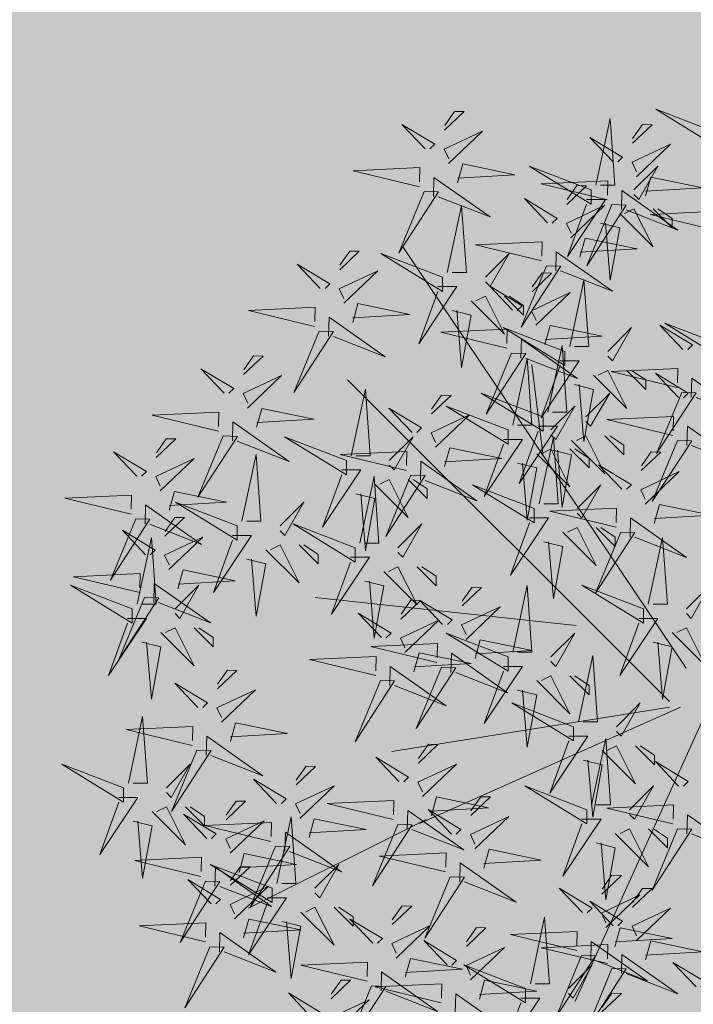
# Model space of a CAD drawing. Units: inches. Extents: x 1704 to 6393, y -157 to 1172.
# Tile 81 of 122: x 2048 to 2064, y 1006 to 1030. Entities that reach past the tile are written whole.
import ezdxf

# ---------------------------------------------------------------- set-up
doc = ezdxf.new("R2010")
doc.units = ezdxf.units.IN
doc.header["$MEASUREMENT"] = 0
doc.layers.add('A-ANNO-DIMS', color=7, linetype='Continuous', lineweight=13)
doc.layers.add('L-shrub', color=74, linetype='Continuous', lineweight=18)
doc.layers.add('L-HRDS-PATT', color=9, linetype='Continuous', lineweight=13, true_color=0xc5c1ba)
doc.styles.get("Standard").update_dxf_attribs({"font": 'arial.ttf'})
doc.dimstyles.get("Standard").update_dxf_attribs({"dimtxt": 6, "dimasz": 2, "dimexe": 0.18, "dimexo": 0.0625, "dimgap": 0.09, "dimtad": 0, "dimtih": 1, "dimtoh": 1, "dimdec": 1, "dimzin": 0, "dimdsep": 46, "dimlunit": 3, "dimtxsty": 'Standard', "dimblk": 'ARCHTICK', "dimcen": 0.09, "dimadec": 0, "dimazin": 0, "dimtfac": 1, "dimtdec": 1, "dimtofl": 0, "dimtmove": 0, "dimatfit": 3, "dimfxl": 1, "dimtolj": 1, "dimtzin": 0, "dimarcsym": 0})

# ---------------------------------------------------------------- blocks, each defined once
blk = doc.blocks.new('shrub3')
for p, q in [((-5.99, -2.5), (58.67, 140.12)), ((130.91, 52.02), (217.13, 95.08)), ((7.48, -2.5), (134.11, 54.01)), ((12.87, -2.5), (147.58, 19.03)), ((12.87, -5.19), (169.14, -161.27)), ((4.78, -21.34), (142.19, -225.85)), ((58.17, -42.16), (184.8, -55.61)), ((74.33, -125.58), (79.72, -168.64))]:
    blk.add_line(p, q)
for points in [[(85.01, 138.66), (75.77, 138.66), (94.24, 166.33), (85.01, 140.97)], [(157.38, 132.76), (169.66, 162.48), (150.47, 132.94), (157.38, 132.76)], [(40.78, 124.29), (53.06, 154.01), (33.87, 124.47), (40.78, 124.29)], [(116.79, 145.77), (116.56, 136.54), (89.36, 155.7), (114.49, 145.83)], [(175.19, 155.2), (158.65, 139.45), (177.32, 148.22), (175.13, 152.89)], [(45.65, 145.34), (36.2, 136.34), (40.81, 136.22), (45.59, 143.03)], [(55.62, 117.94), (67.9, 147.66), (48.71, 118.11), (55.62, 117.94)], [(152.83, 135.19), (152.6, 125.95), (125.4, 145.11), (150.53, 135.24)], [(186.54, 147.99), (197.78, 136.16), (181.88, 145.8), (184.24, 148.05)], [(235.82, 113.71), (248.1, 143.42), (228.91, 113.88), (235.82, 113.71)], [(61.92, 134.05), (50.38, 122.52), (59.61, 138.66), (61.92, 136.35)], [(105.09, 139.14), (102.56, 129.96), (77.32, 135.21), (105.04, 136.83)], [(82.7, 134.05), (112.71, 122.52), (82.7, 140.97), (82.7, 134.05)], [(123.59, 140.98), (155.69, 133.25), (123.36, 131.75), (123.53, 138.68)], [(177.09, 138.99), (167.64, 129.99), (172.25, 129.87), (177.04, 136.68)], [(36.23, 126.72), (36, 117.49), (8.8, 136.64), (33.93, 126.77)], [(-0.02, 133.17), (11.22, 121.34), (-4.68, 130.97), (-2.32, 133.22)], [(51.07, 120.36), (50.84, 111.13), (23.64, 130.29), (48.77, 120.42)], [(80.39, 131.74), (73.46, 99.46), (71.15, 131.74), (78.08, 131.74)], [(109.47, 129.79), (92.93, 114.04), (111.6, 122.81), (109.41, 127.48)], [(159.63, 130.4), (191.73, 122.67), (159.4, 121.17), (159.57, 128.09)], [(201.04, 101.49), (191.81, 103.79), (196.42, 129.16), (198.73, 101.49)], [(141.13, 128.55), (138.6, 119.38), (113.36, 124.63), (141.08, 126.24)], [(231.27, 116.13), (231.04, 106.9), (203.84, 126.05), (228.97, 116.19)], [(24.53, 120.08), (22, 110.91), (-3.24, 116.16), (24.47, 117.77)], [(43.03, 121.93), (75.13, 114.2), (42.8, 112.7), (42.97, 119.62)], [(120.82, 122.58), (132.06, 110.75), (116.16, 120.39), (118.52, 122.64)], [(57.87, 115.58), (89.97, 107.84), (57.64, 106.34), (57.81, 113.27)], [(145.51, 119.2), (128.97, 103.45), (147.64, 112.22), (145.45, 116.9)], [(207.97, 89.96), (198.73, 89.96), (217.2, 117.63), (207.97, 92.27)], [(39.37, 113.73), (36.84, 104.56), (11.6, 109.81), (39.31, 111.42)], [(28.91, 110.73), (12.37, 94.98), (31.04, 103.75), (28.85, 108.43)], [(111.37, 113.58), (101.92, 104.58), (106.53, 104.46), (111.31, 111.27)], [(156.86, 111.99), (168.1, 100.16), (152.2, 109.8), (154.56, 112.05)], [(191.81, 96.88), (175.65, 113.02), (184.88, 94.57), (189.5, 96.88)], [(237.94, 81.95), (250.22, 111.66), (231.03, 82.12), (237.94, 81.95)], [(238.07, 111.34), (270.17, 103.61), (237.84, 102.11), (238.01, 109.03)], [(119.22, 79.83), (131.5, 109.54), (112.31, 80), (119.22, 79.83)], [(219.57, 109.49), (217.04, 100.32), (191.8, 105.57), (219.52, 107.19)], [(43.75, 104.38), (27.21, 88.63), (45.88, 97.4), (43.69, 102.07)], [(40.26, 103.52), (51.5, 91.69), (35.6, 101.33), (37.96, 103.58)], [(147.41, 102.99), (137.96, 93.99), (142.57, 93.88), (147.36, 100.68)], [(175.65, 94.57), (166.41, 103.79), (166.41, 99.18), (173.34, 94.57)], [(55.1, 97.17), (66.34, 85.34), (50.44, 94.98), (52.8, 97.23)], [(223.95, 100.15), (207.41, 84.4), (226.08, 93.17), (223.89, 97.84)], [(30.81, 94.52), (21.36, 85.52), (25.97, 85.41), (30.75, 92.21)], [(48.4, 63.38), (39.16, 65.68), (43.78, 91.04), (46.09, 63.38)], [(114.67, 82.25), (114.44, 73.02), (87.24, 92.18), (112.37, 82.31)], [(204.02, 65.01), (216.3, 94.72), (197.11, 65.18), (204.02, 65.01)], [(205.66, 85.35), (235.67, 73.82), (205.66, 92.27), (205.66, 85.35)], [(233.39, 84.37), (233.16, 75.14), (205.96, 94.29), (231.09, 84.43)], [(235.3, 92.94), (246.54, 81.11), (230.64, 90.74), (233, 92.99)], [(8.98, 56.54), (21.26, 86.25), (2.07, 56.71), (8.98, 56.54)], [(45.65, 88.17), (36.2, 79.17), (40.81, 79.05), (45.59, 85.86)], [(184.88, 85.35), (173.34, 73.82), (182.57, 89.96), (184.88, 87.65)], [(144.66, 54.42), (156.94, 84.13), (137.75, 54.59), (144.66, 54.42)], [(203.35, 83.04), (196.42, 50.76), (194.11, 83.04), (201.04, 83.04)], [(225.85, 83.93), (216.4, 74.93), (221.01, 74.82), (225.8, 81.63)], [(55.33, 51.85), (46.09, 51.85), (64.56, 79.52), (55.33, 54.15)], [(121.47, 77.46), (153.57, 69.73), (121.24, 68.23), (121.41, 75.15)], [(199.47, 67.43), (199.24, 58.2), (172.04, 77.35), (197.17, 67.49)], [(221.69, 77.73), (219.16, 68.56), (193.92, 73.81), (221.64, 75.43)], [(240.19, 79.58), (272.29, 71.85), (239.96, 70.35), (240.13, 77.27)], [(273.12, 52.79), (263.89, 55.09), (268.5, 80.46), (270.81, 52.79)], [(39.16, 58.76), (23, 74.9), (32.24, 56.46), (36.86, 58.76)], [(102.97, 75.62), (100.44, 66.44), (75.2, 71.69), (102.92, 73.31)], [(4.43, 58.96), (4.2, 49.73), (-23, 68.88), (2.13, 59.02)], [(226.07, 68.39), (209.53, 52.64), (228.2, 61.41), (226.01, 66.08)], [(280.05, 41.26), (270.81, 41.26), (289.28, 68.93), (280.05, 43.57)], [(23, 56.46), (13.77, 65.68), (13.77, 61.07), (20.7, 56.46)], [(107.35, 66.27), (90.81, 50.52), (109.48, 59.29), (107.29, 63.96)], [(140.11, 56.84), (139.88, 47.61), (112.68, 66.77), (137.81, 56.9)], [(206.27, 62.64), (238.37, 54.91), (206.04, 53.41), (206.21, 60.33)], [(263.89, 48.18), (247.73, 64.32), (256.96, 45.87), (261.58, 48.18)], [(118.7, 59.06), (129.94, 47.23), (114.04, 56.86), (116.4, 59.12)], [(187.77, 60.79), (185.24, 51.62), (160, 56.87), (187.72, 58.49)], [(237.42, 61.17), (248.66, 49.35), (232.76, 58.98), (235.12, 61.23)], [(11.23, 54.17), (43.33, 46.44), (11, 44.94), (11.17, 51.86)], [(53.02, 47.24), (83.03, 35.71), (53.02, 54.15), (53.02, 47.24)], [(247.73, 45.87), (238.49, 55.09), (238.49, 50.48), (245.42, 45.87)], [(32.24, 47.24), (20.7, 35.71), (29.93, 51.85), (32.24, 49.54)], [(54.76, 23.15), (45.52, 25.45), (50.14, 50.81), (52.45, 23.15)], [(109.25, 50.06), (99.8, 41.06), (104.41, 40.94), (109.19, 47.75)], [(128.41, 50.21), (125.88, 41.03), (100.64, 46.28), (128.36, 47.9)], [(146.91, 52.05), (179.01, 44.32), (146.68, 42.82), (146.85, 49.75)], [(192.15, 51.45), (175.61, 35.7), (194.28, 44.47), (192.09, 49.14)], [(227.97, 52.17), (218.52, 43.17), (223.13, 43.06), (227.92, 49.87)], [(242.18, 18.42), (254.46, 48.14), (235.27, 18.6), (242.18, 18.42)], [(50.71, 44.93), (43.78, 12.65), (41.47, 44.93), (48.4, 44.93)], [(203.5, 44.24), (214.74, 32.41), (198.84, 42.04), (201.2, 44.29)], [(277.74, 36.65), (307.75, 25.12), (277.74, 43.57), (277.74, 36.65)], [(61.69, 11.62), (52.45, 11.62), (70.92, 39.29), (61.69, 13.92)], [(132.79, 40.86), (116.25, 25.11), (134.92, 33.88), (132.73, 38.55)], [(256.96, 36.65), (245.42, 25.12), (254.65, 41.26), (256.96, 38.95)], [(8.46, 35.77), (19.7, 23.94), (3.8, 33.57), (6.16, 35.82)], [(45.52, 18.53), (29.36, 34.67), (38.6, 16.23), (43.22, 18.53)], [(144.14, 33.65), (155.38, 21.82), (139.48, 31.46), (141.84, 33.71)], [(194.05, 35.23), (184.6, 26.23), (189.21, 26.12), (194, 32.93)], [(275.43, 34.34), (268.5, 2.06), (266.19, 34.34), (273.12, 34.34)], [(237.63, 20.85), (237.4, 11.62), (210.2, 30.77), (235.33, 20.91)], [(29.36, 16.23), (20.13, 25.45), (20.13, 20.84), (27.06, 16.23)], [(134.69, 24.65), (125.24, 15.65), (129.85, 15.53), (134.63, 22.34)], [(86.56, -10.73), (77.32, -8.43), (81.94, 16.94), (84.25, -10.73)], [(244.43, 16.06), (276.53, 8.33), (244.2, 6.83), (244.37, 13.75)], [(38.6, 7), (27.06, -4.52), (36.29, 11.62), (38.6, 9.31)], [(59.38, 7), (89.39, -4.52), (59.38, 13.92), (59.38, 7)], [(153.14, -15.45), (165.42, 14.26), (146.23, -15.28), (153.14, -15.45)], [(225.93, 14.21), (223.4, 5.04), (198.16, 10.29), (225.88, 11.9)], [(93.49, -22.26), (84.25, -22.26), (102.72, 5.41), (93.49, -19.96)], [(123.46, -21.81), (135.74, 7.91), (116.55, -21.63), (123.46, -21.81)], [(230.31, 4.87), (213.77, -10.89), (232.44, -2.12), (230.25, 2.56)], [(57.07, 4.7), (50.14, -27.58), (47.83, 4.7), (54.76, 4.7)], [(77.32, -15.34), (61.16, 0.8), (70.4, -17.65), (75.02, -15.34)], [(148.59, -13.03), (148.36, -22.26), (121.16, -3.11), (146.29, -12.97)], [(241.66, -2.35), (252.9, -14.18), (237, -4.54), (239.36, -2.29)], [(20.84, -34.02), (11.6, -31.72), (16.22, -6.36), (18.53, -34.02)], [(61.16, -17.65), (51.93, -8.43), (51.93, -13.04), (58.86, -17.65)], [(118.91, -19.38), (118.68, -28.61), (91.48, -9.46), (116.61, -19.33)], [(268.88, -34.02), (259.65, -31.72), (264.26, -6.36), (266.57, -34.02)], [(232.21, -11.35), (222.76, -20.35), (227.37, -20.46), (232.16, -13.66)], [(27.76, -45.55), (18.53, -45.55), (37, -17.88), (27.76, -43.25)], [(155.39, -17.82), (187.49, -25.55), (155.16, -27.05), (155.33, -20.13)], [(275.81, -45.55), (266.57, -45.55), (285.04, -17.88), (275.81, -43.25)], [(11.6, -38.64), (-4.56, -22.5), (4.68, -40.94), (9.3, -38.64)], [(70.4, -26.87), (58.86, -38.4), (68.09, -22.26), (70.4, -24.57)], [(91.18, -26.87), (121.19, -38.4), (91.18, -19.96), (91.18, -26.87)], [(136.89, -19.67), (134.36, -28.84), (109.12, -23.59), (136.84, -21.97)], [(259.65, -38.64), (243.49, -22.5), (252.72, -40.94), (257.34, -38.64)], [(107.21, -26.02), (104.68, -35.19), (79.44, -29.94), (107.16, -28.33)], [(125.71, -24.17), (157.81, -31.9), (125.48, -33.4), (125.65, -26.48)], [(267.62, -55.68), (279.9, -25.97), (260.71, -55.51), (267.62, -55.68)], [(88.87, -29.18), (81.94, -61.46), (79.63, -29.18), (86.56, -29.18)], [(141.27, -29.01), (124.73, -44.76), (143.4, -35.99), (141.21, -31.32)], [(243.49, -40.94), (234.25, -31.72), (234.25, -36.33), (241.18, -40.94)], [(111.59, -35.37), (95.05, -51.12), (113.72, -42.35), (111.53, -37.67)], [(152.62, -36.23), (163.86, -48.05), (147.96, -38.42), (150.32, -36.17)], [(160.76, -63.67), (151.53, -61.36), (156.14, -36), (158.45, -63.67)], [(122.94, -42.58), (134.18, -54.41), (118.28, -44.77), (120.64, -42.52)], [(4.68, -50.16), (-6.86, -61.69), (2.37, -45.55), (4.68, -47.86)], [(25.46, -50.16), (55.47, -61.69), (25.46, -43.25), (25.46, -50.16)], [(143.17, -45.23), (133.72, -54.23), (138.33, -54.34), (143.12, -47.53)], [(167.69, -75.2), (158.45, -75.2), (176.92, -47.53), (167.69, -72.89)], [(218, -74.25), (208.77, -71.95), (213.38, -46.59), (215.69, -74.25)], [(263.07, -53.26), (262.84, -62.49), (235.64, -43.34), (260.77, -53.2)], [(252.72, -50.16), (241.18, -61.69), (250.41, -45.55), (252.72, -47.86)], [(273.5, -50.16), (303.51, -61.69), (273.5, -43.25), (273.5, -50.16)], [(23.15, -52.47), (16.22, -84.75), (13.91, -52.47), (20.84, -52.47)], [(113.49, -51.58), (104.04, -60.58), (108.65, -60.69), (113.43, -53.89)], [(151.53, -68.28), (135.37, -52.14), (144.6, -70.59), (149.22, -68.28)], [(271.19, -52.47), (264.26, -84.75), (261.95, -52.47), (268.88, -52.47)], [(73.84, -82.72), (64.6, -80.42), (69.22, -55.06), (71.53, -82.72)], [(36.54, -87.45), (48.82, -57.73), (29.63, -87.27), (36.54, -87.45)], [(135.37, -70.59), (126.13, -61.36), (126.13, -65.97), (133.06, -70.59)], [(224.93, -85.78), (215.69, -85.78), (234.16, -58.11), (224.93, -83.48)], [(251.37, -59.9), (248.84, -69.07), (223.6, -63.82), (251.32, -62.2)], [(269.87, -58.05), (301.97, -65.78), (269.64, -67.28), (269.81, -60.36)], [(80.77, -94.25), (71.53, -94.25), (90, -66.58), (80.77, -91.95)], [(208.77, -78.87), (192.61, -62.73), (201.84, -81.17), (206.46, -78.87)], [(271.86, -93.8), (284.14, -64.08), (264.95, -93.62), (271.86, -93.8)], [(64.6, -87.34), (48.44, -71.2), (57.68, -89.64), (62.3, -87.34)], [(255.75, -69.24), (239.21, -85), (257.88, -76.23), (255.7, -71.55)], [(31.99, -85.02), (31.76, -94.25), (4.56, -75.1), (29.69, -84.96)], [(144.6, -79.81), (133.06, -91.34), (142.29, -75.2), (144.6, -77.5)], [(165.38, -79.81), (195.39, -91.34), (165.38, -72.89), (165.38, -79.81)], [(192.61, -81.17), (183.37, -71.95), (183.37, -76.56), (190.3, -81.17)], [(267.1, -76.46), (278.34, -88.28), (262.44, -78.65), (264.8, -76.4)], [(48.44, -89.64), (39.21, -80.42), (39.21, -85.03), (46.14, -89.64)], [(165, -106.02), (155.77, -103.71), (160.38, -78.35), (162.69, -106.02)], [(138.3, -114.97), (150.58, -85.26), (131.39, -114.8), (138.3, -114.97)], [(163.07, -82.11), (156.14, -114.39), (153.83, -82.11), (160.76, -82.11)], [(201.84, -90.4), (190.3, -101.92), (199.53, -85.78), (201.84, -88.09)], [(222.62, -90.4), (252.63, -101.92), (222.62, -83.48), (222.62, -90.4)], [(267.31, -91.37), (267.08, -100.61), (239.88, -81.45), (265.01, -91.32)], [(257.65, -85.46), (248.2, -94.46), (252.81, -94.57), (257.6, -87.76)], [(38.79, -89.81), (70.89, -97.54), (38.56, -99.04), (38.73, -92.12)], [(171.93, -117.54), (162.69, -117.54), (181.16, -89.88), (171.93, -115.24)], [(20.29, -91.66), (17.76, -100.83), (-7.48, -95.58), (20.23, -93.97)], [(57.68, -98.86), (46.14, -110.39), (55.37, -94.25), (57.68, -96.56)], [(86.56, -120.84), (77.32, -118.53), (81.94, -93.17), (84.25, -120.84)], [(78.46, -98.86), (108.47, -110.39), (78.46, -91.95), (78.46, -98.86)], [(155.77, -110.63), (139.61, -94.49), (148.84, -112.93), (153.46, -110.63)], [(220.31, -92.7), (213.38, -124.98), (211.07, -92.7), (218, -92.7)], [(69.6, -127.19), (60.36, -124.88), (64.98, -99.52), (67.29, -127.19)], [(255.61, -98.01), (253.08, -107.18), (227.84, -101.93), (255.56, -100.32)], [(274.11, -96.16), (306.21, -103.89), (273.88, -105.4), (274.05, -98.47)], [(8.98, -131.91), (21.26, -102.2), (2.07, -131.74), (8.98, -131.91)], [(24.67, -101), (8.13, -116.76), (26.8, -107.99), (24.61, -103.31)], [(76.15, -101.17), (69.22, -133.45), (66.91, -101.17), (73.84, -101.17)], [(93.49, -132.37), (84.25, -132.37), (102.72, -104.7), (93.49, -130.06)], [(133.75, -112.55), (133.52, -121.78), (106.32, -102.62), (131.45, -112.49)], [(139.61, -112.93), (130.37, -103.71), (130.37, -108.32), (137.3, -112.93)], [(229.46, -134.03), (241.74, -104.31), (222.55, -133.86), (229.46, -134.03)], [(36.02, -108.22), (47.26, -120.04), (31.36, -110.41), (33.72, -108.16)], [(77.32, -125.45), (61.16, -109.31), (70.4, -127.75), (75.02, -125.45)], [(259.99, -107.36), (243.45, -123.11), (262.12, -114.34), (259.94, -109.66)], [(76.53, -138.72), (67.29, -138.72), (85.76, -111.05), (76.53, -136.41)], [(271.34, -114.57), (282.58, -126.4), (266.68, -116.76), (269.04, -114.51)], [(26.57, -117.22), (17.12, -126.22), (21.73, -126.33), (26.51, -119.53)], [(60.36, -131.8), (44.2, -115.66), (53.44, -134.11), (58.06, -131.8)], [(61.16, -127.75), (51.93, -118.53), (51.93, -123.14), (58.86, -127.75)], [(122.05, -119.18), (119.52, -128.36), (94.28, -123.11), (122, -121.49)], [(148.84, -122.16), (137.3, -133.69), (146.53, -117.54), (148.84, -119.85)], [(140.55, -117.34), (172.65, -125.07), (140.32, -126.57), (140.49, -119.65)], [(169.62, -122.16), (199.63, -133.69), (169.62, -115.24), (169.62, -122.16)], [(4.43, -129.49), (4.2, -138.72), (-23, -119.56), (2.13, -129.43)], [(224.91, -131.61), (224.68, -140.84), (197.48, -121.68), (222.61, -131.55)], [(261.89, -123.57), (252.44, -132.57), (257.05, -132.69), (261.84, -125.88)], [(6.86, -155.2), (19.14, -125.49), (-0.05, -155.03), (6.86, -155.2)], [(44.2, -134.11), (34.97, -124.88), (34.97, -129.5), (41.9, -134.11)], [(126.43, -128.53), (109.89, -144.28), (128.56, -135.51), (126.37, -130.84)], [(167.31, -124.46), (160.38, -156.74), (158.07, -124.46), (165, -124.46)], [(59, -158.95), (49.76, -156.64), (54.38, -131.28), (56.69, -158.95)], [(70.4, -136.98), (58.86, -148.51), (68.09, -132.37), (70.4, -134.67)], [(91.18, -136.98), (121.19, -148.51), (91.18, -130.06), (91.18, -136.98)], [(11.23, -134.28), (43.33, -142.01), (11, -143.51), (11.17, -136.58)], [(74.22, -143.33), (104.23, -154.86), (74.22, -136.41), (74.22, -143.33)], [(137.78, -135.74), (149.02, -147.57), (133.12, -137.94), (135.48, -135.69)], [(213.21, -138.24), (210.68, -147.41), (185.44, -142.16), (213.16, -140.55)], [(231.71, -136.39), (263.81, -144.13), (231.48, -145.63), (231.65, -138.7)], [(2.31, -152.78), (2.08, -162.01), (-25.12, -142.86), (0.01, -152.72)], [(53.44, -143.33), (41.9, -154.86), (51.13, -138.72), (53.44, -141.02)], [(65.93, -170.48), (56.69, -170.48), (75.16, -142.81), (65.93, -168.17)], [(88.87, -139.28), (81.94, -171.56), (79.63, -139.28), (86.56, -139.28)], [(49.76, -163.56), (33.6, -147.42), (42.84, -165.87), (47.46, -163.56)], [(71.91, -145.64), (64.98, -177.92), (62.67, -145.64), (69.6, -145.64)], [(89.54, -174.26), (101.82, -144.54), (82.63, -174.09), (89.54, -174.26)], [(128.33, -144.74), (118.88, -153.74), (123.49, -153.86), (128.27, -147.05)], [(217.59, -147.59), (201.05, -163.34), (219.72, -154.57), (217.53, -149.9)], [(8.46, -152.68), (19.7, -164.51), (3.8, -154.87), (6.16, -152.62)], [(9.11, -157.57), (41.21, -165.3), (8.88, -166.8), (9.05, -159.88)], [(33.6, -165.87), (24.37, -156.64), (24.37, -161.26), (31.3, -165.87)], [(182.82, -184.85), (195.1, -155.13), (175.91, -184.67), (182.82, -184.85)], [(228.94, -154.8), (240.18, -166.63), (224.28, -156.99), (226.64, -154.74)], [(84.99, -171.84), (84.76, -181.07), (57.56, -161.91), (82.69, -171.78)], [(219.49, -163.8), (210.04, -172.8), (214.65, -172.92), (219.44, -166.11)], [(-14.82, -177.21), (15.19, -188.74), (-14.82, -170.29), (-14.82, -177.21)], [(42.84, -175.09), (31.3, -186.62), (40.53, -170.48), (42.84, -172.79)], [(63.62, -175.09), (93.63, -186.62), (63.62, -168.17), (63.62, -175.09)], [(118.36, -194.95), (109.13, -192.64), (113.74, -167.28), (116.05, -194.95)], [(6.34, -175.97), (17.58, -187.8), (1.68, -178.17), (4.04, -175.92)], [(91.79, -176.62), (123.89, -184.36), (91.56, -185.86), (91.73, -178.93)], [(178.27, -182.42), (178.04, -191.65), (150.84, -172.5), (175.97, -182.36)], [(73.29, -178.47), (70.76, -187.64), (45.52, -182.39), (73.23, -180.78)], [(61.31, -177.4), (54.38, -209.68), (52.07, -177.4), (59, -177.4)], [(125.29, -206.48), (116.05, -206.48), (134.52, -178.81), (125.29, -204.17)], [(109.13, -199.56), (92.96, -183.42), (102.2, -201.86), (106.82, -199.56)], [(77.67, -187.82), (61.13, -203.57), (79.8, -194.8), (77.61, -190.13)], [(72.58, -216.61), (84.86, -186.89), (65.67, -216.43), (72.58, -216.61)], [(166.57, -189.06), (164.04, -198.23), (138.8, -192.98), (166.52, -191.37)], [(185.07, -187.21), (217.17, -194.94), (184.84, -196.44), (185.01, -189.52)], [(92.96, -201.86), (83.73, -192.64), (83.73, -197.25), (90.66, -201.86)], [(89.02, -195.03), (100.26, -206.86), (84.36, -197.22), (86.72, -194.97)], [(170.95, -198.4), (154.41, -214.16), (173.08, -205.39), (170.89, -200.71)], [(68.03, -214.18), (67.8, -223.42), (40.6, -204.26), (65.73, -214.13)], [(79.57, -204.03), (70.12, -213.03), (74.73, -213.15), (79.51, -206.34)], [(122.98, -211.09), (152.99, -222.62), (122.98, -204.17), (122.98, -211.09)], [(46.28, -237.29), (37.04, -234.99), (41.66, -209.63), (43.97, -237.29)], [(102.2, -211.09), (90.66, -222.62), (99.89, -206.48), (102.2, -208.78)], [(182.3, -205.62), (193.54, -217.44), (177.64, -207.81), (180, -205.56)], [(120.67, -213.39), (113.74, -245.67), (111.43, -213.39), (118.36, -213.39)], [(172.85, -214.62), (163.4, -223.62), (168.01, -223.73), (172.8, -216.93)], [(40.78, -246.25), (53.06, -216.54), (33.87, -246.08), (40.78, -246.25)], [(74.83, -218.97), (106.93, -226.7), (74.6, -228.2), (74.77, -221.28)], [(56.33, -220.82), (53.8, -229.99), (28.56, -224.74), (56.27, -223.13)], [(53.21, -248.82), (43.97, -248.82), (62.44, -221.15), (53.21, -246.52)], [(131.94, -252.6), (144.22, -222.89), (125.03, -252.43), (131.94, -252.6)], [(37.04, -241.91), (20.88, -225.77), (30.12, -244.21), (34.74, -241.91)], [(-9.97, -233.79), (22.13, -241.53), (-10.2, -243.03), (-10.03, -236.1)], [(36.23, -243.83), (36, -253.06), (8.8, -233.9), (33.93, -243.77)], [(60.71, -230.17), (44.17, -245.92), (62.84, -237.15), (60.65, -232.47)], [(20.88, -244.21), (11.65, -234.99), (11.65, -239.6), (18.58, -244.21)], [(72.06, -237.38), (83.3, -249.21), (67.4, -239.57), (69.76, -237.32)], [(127.39, -250.18), (127.16, -259.41), (99.96, -240.26), (125.09, -250.12)], [(50.9, -253.43), (80.91, -264.96), (50.9, -246.52), (50.9, -253.43)], [(62.61, -246.38), (53.16, -255.38), (57.77, -255.49), (62.55, -248.69)], [(24.53, -250.46), (22, -259.64), (-3.24, -254.39), (24.47, -252.77)], [(30.12, -253.43), (18.58, -264.96), (27.81, -248.82), (30.12, -251.13)], [(43.03, -248.62), (75.13, -256.35), (42.8, -257.85), (42.97, -250.92)], [(48.59, -255.74), (41.66, -288.02), (39.35, -255.74), (46.28, -255.74)], [(115.69, -256.81), (113.16, -265.99), (87.92, -260.74), (115.64, -259.12)], [(134.19, -254.97), (166.29, -262.7), (133.96, -264.2), (134.13, -257.28)], [(28.91, -259.81), (12.37, -275.56), (31.04, -266.79), (28.85, -262.12)], [(40.26, -267.02), (51.5, -278.85), (35.6, -269.21), (37.96, -266.96)], [(120.07, -266.16), (103.53, -281.91), (122.2, -273.14), (120.01, -268.47)], [(-10.58, -280.96), (19.43, -292.49), (-10.58, -274.04), (-10.58, -280.96)], [(30.81, -276.02), (21.36, -285.02), (25.97, -285.14), (30.75, -278.33)], [(131.42, -273.37), (142.66, -285.2), (126.76, -275.57), (129.12, -273.32)], [(121.97, -282.37), (112.52, -291.38), (117.13, -291.49), (121.91, -284.68)]]:
    blk.add_lwpolyline(points)
blk = doc.blocks.new('_ArchTick')
at = {"color": 0, "linetype": 'ByBlock', "const_width": 0.15}
blk.add_lwpolyline([(-0.5, -0.5), (0.5, 0.5)], dxfattribs=at)
blk = doc.blocks.new('*D94')
at = {"layer": 'A-ANNO-DIMS', "color": 0, "lineweight": -2, "transparency": 16777216}
for p, q in [((1898.349, 895.275), (1898.349, 1105.287)), ((2073.349, 895.275), (2073.349, 1105.287)), ((1898.349, 1105.107), (1979.39, 1105.107)), ((2073.349, 1105.107), (1992.307, 1105.107))]:
    blk.add_line(p, q, dxfattribs=at)
at = {"layer": 'Defpoints', "color": 0, "lineweight": -3, "transparency": 16777216}
for p in [(2073.349, 1105.107), (1898.349, 895.213), (2073.349, 895.213)]:
    blk.add_point(p, dxfattribs=at)
at = {"layer": 'A-ANNO-DIMS', "color": 0, "lineweight": -2, "transparency": 16777216, "xscale": 2, "yscale": 2, "zscale": 2, "rotation": 180}
blk.add_blockref('_ArchTick', (1898.349, 1105.107), dxfattribs=at)
at = {"layer": 'A-ANNO-DIMS', "color": 0, "lineweight": -2, "transparency": 16777216, "xscale": 2, "yscale": 2, "zscale": 2}
blk.add_blockref('_ArchTick', (2073.349, 1105.107), dxfattribs=at)
at = {"layer": 'A-ANNO-DIMS', "color": 0, "transparency": 16777216, "insert": (1985.849, 1105.107), "char_height": 6, "attachment_point": 5}
blk.add_mtext('\\A1;175', dxfattribs=at)

msp = doc.modelspace()

# ---------------------------------------------------------------- hatches: boundary and pattern name
at = {"layer": 'L-HRDS-PATT', "transparency": 33554643}
h = msp.add_hatch(color=256, dxfattribs=at)
h.dxf.hatch_style = 1
h.paths.add_polyline_path([(2065.589, 1033.213), (1898.349, 1033.213), (1898.349, 895.213), (2065.589, 895.213)])

# ---------------------------------------------------------------- block references
at = {"layer": 'L-shrub', "xscale": 0.0510581485411622, "yscale": 0.0510581485411622, "zscale": 0.0510581485411622, "rotation": 180}
msp.add_blockref('shrub3', (2064.28, 1012.986), dxfattribs=at)

# ---------------------------------------------------------------- dimensions: what is measured, and where the dimension line sits
at = {"layer": 'A-ANNO-DIMS'}
dim = msp.add_linear_dim(base=(2073.349, 1105.107), p1=(1898.349, 895.213), p2=(2073.349, 895.213), dimstyle='Standard', override={"dimdec": 0, "dimlfac": 1, "dimrnd": 0, "dimzin": 0, "dimdsep": 46, "dimlunit": 2}, dxfattribs=at)
dim.commit()
dim.dimension.update_dxf_attribs({"geometry": '*D94', "text_midpoint": (1985.849, 1105.107)})

doc.saveas('drawing.dxf')
